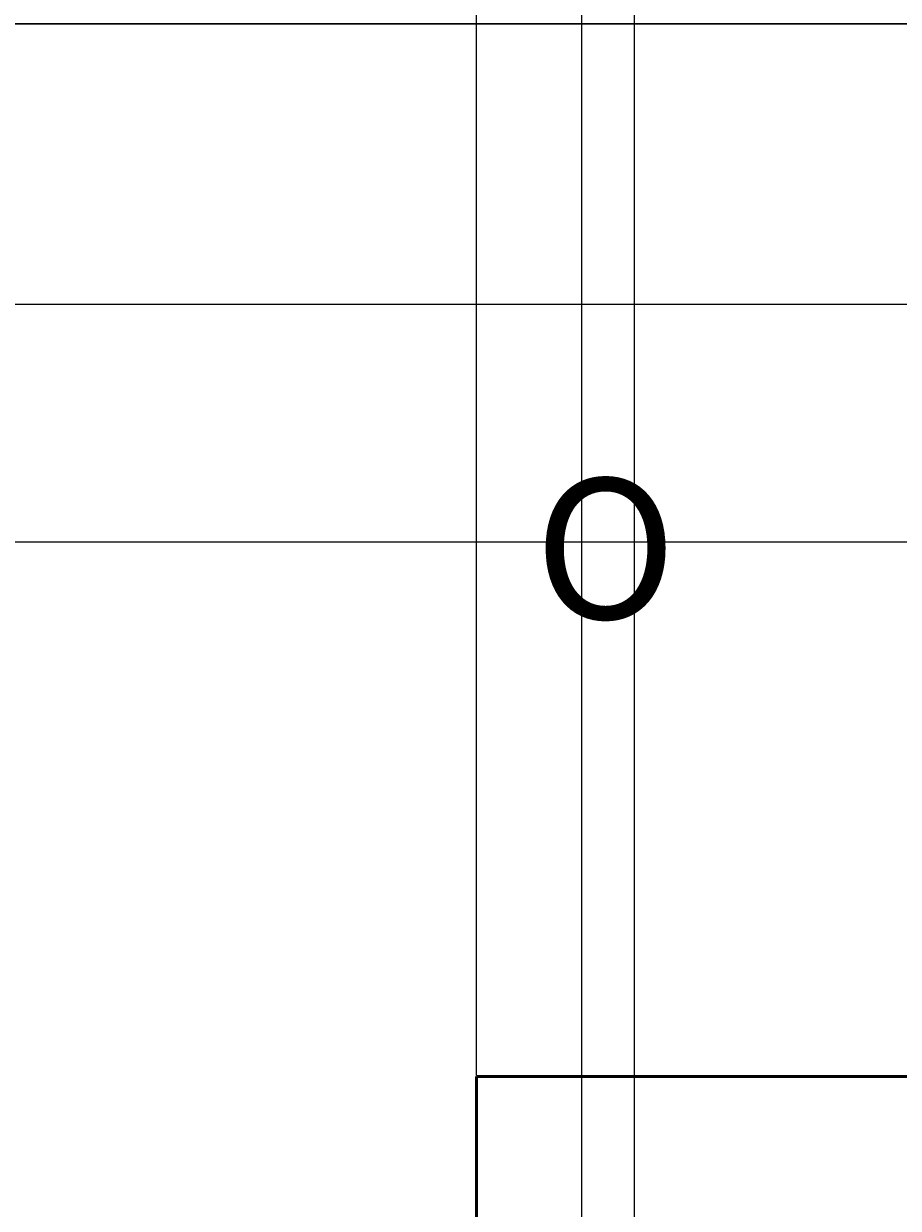
# Model space of a CAD drawing. Units: inches. Extents: x 37 to 824, y -700 to 234.
# Tile 63 of 77: x 264 to 314, y 8 to 75. Entities that reach past the tile are written whole.
import ezdxf

# ---------------------------------------------------------------- set-up
doc = ezdxf.new("R2010")
doc.units = ezdxf.units.IN
doc.header["$MEASUREMENT"] = 0
for name, color, linetype, lineweight in [('A-ANNO-DIMS', 2, 'Continuous', 18), ('A-ANNO-TEXT', 7, 'Continuous', 18), ('A-WALL', 2, 'Continuous', 50)]:
    doc.layers.add(name, color=color, linetype=linetype, lineweight=lineweight)
doc.styles.get("Standard").update_dxf_attribs({"font": 'arial.ttf'})
doc.dimstyles.get("Standard").update_dxf_attribs({"dimtxt": 0.18, "dimasz": 0.18, "dimexe": 0.18, "dimexo": 0.0625, "dimgap": 0.09, "dimtad": 0, "dimtih": 1, "dimtoh": 1, "dimdec": 1, "dimzin": 0, "dimdsep": 46, "dimlunit": 4, "dimtxsty": 'Standard', "dimcen": 0.09, "dimadec": 0, "dimazin": 0, "dimtfac": 1, "dimtdec": 1, "dimtofl": 0, "dimtmove": 0, "dimatfit": 3, "dimfxl": 1, "dimtolj": 1, "dimtzin": 0, "dimarcsym": 0})

# ---------------------------------------------------------------- blocks, each defined once
blk = doc.blocks.new('*D61')
at = {"layer": 'A-ANNO-DIMS', "color": 0, "lineweight": -2, "ltscale": 0.5, "transparency": 16777216}
for p, q in [((419.015, 75.09), (78.159, 75.09)), ((78.339, 74.91), (78.339, 67.271)), ((78.339, 59.27), (78.339, 66.91)), ((419.015, 59.09), (78.159, 59.09))]:
    blk.add_line(p, q, dxfattribs=at)
at = {"layer": 'A-ANNO-DIMS', "color": 0, "ltscale": 0.5, "transparency": 16777216}
for points in [[(78.309, 74.91), (78.369, 74.91), (78.339, 75.09)], [(78.309, 59.27), (78.369, 59.27), (78.339, 59.09)]]:
    blk.add_solid(points, dxfattribs=at)
at = {"layer": 'Defpoints', "color": 0, "ltscale": 0.5, "transparency": 16777216}
for p in [(419.077, 75.09), (78.339, 59.09), (419.077, 59.09)]:
    blk.add_point(p, dxfattribs=at)
at = {"layer": 'A-ANNO-DIMS', "color": 0, "ltscale": 0.5, "transparency": 16777216, "insert": (78.339, 67.09), "char_height": 0.18, "attachment_point": 5}
blk.add_mtext('\\A1;1\'-4"', dxfattribs=at)
blk = doc.blocks.new('*D76')
at = {"layer": 'A-ANNO-DIMS', "color": 0, "lineweight": -2, "ltscale": 0.5, "transparency": 16777216}
for p, q in [((227.14, 75.09), (513.773, 75.09)), ((513.593, 74.91), (513.593, 60.51)), ((513.593, 45.743), (513.593, 60.144)), ((227.14, 45.563), (513.773, 45.563))]:
    blk.add_line(p, q, dxfattribs=at)
at = {"layer": 'A-ANNO-DIMS', "color": 0, "ltscale": 0.5, "transparency": 16777216}
for points in [[(513.563, 74.91), (513.623, 74.91), (513.593, 75.09)], [(513.563, 45.743), (513.623, 45.743), (513.593, 45.563)]]:
    blk.add_solid(points, dxfattribs=at)
at = {"layer": 'Defpoints', "color": 0, "ltscale": 0.5, "transparency": 16777216}
for p in [(227.077, 75.09), (227.077, 45.563), (513.593, 45.563)]:
    blk.add_point(p, dxfattribs=at)
at = {"layer": 'A-ANNO-DIMS', "color": 0, "ltscale": 0.5, "transparency": 16777216, "insert": (513.593, 60.327), "char_height": 0.18, "attachment_point": 5}
blk.add_mtext('\\A1;2\'-5 1/2"', dxfattribs=at)
blk = doc.blocks.new('*D77')
at = {"layer": 'A-ANNO-DIMS', "color": 0, "lineweight": -2, "ltscale": 0.5, "transparency": 16777216}
for p, q in [((227.077, 45.5), (227.077, -400.406)), ((290.077, 15.028), (290.077, -400.406)), ((227.257, -400.226), (258.248, -400.226)), ((289.897, -400.226), (258.906, -400.226))]:
    blk.add_line(p, q, dxfattribs=at)
at = {"layer": 'A-ANNO-DIMS', "color": 0, "ltscale": 0.5, "transparency": 16777216}
for points in [[(227.257, -400.196), (227.257, -400.256), (227.077, -400.226)], [(289.897, -400.196), (289.897, -400.256), (290.077, -400.226)]]:
    blk.add_solid(points, dxfattribs=at)
at = {"layer": 'Defpoints', "color": 0, "ltscale": 0.5, "transparency": 16777216}
for p in [(227.077, 45.563), (290.077, 15.09), (290.077, -400.226)]:
    blk.add_point(p, dxfattribs=at)
at = {"layer": 'A-ANNO-DIMS', "color": 0, "ltscale": 0.5, "transparency": 16777216, "insert": (258.577, -400.226), "char_height": 0.18, "attachment_point": 5}
blk.add_mtext('\\A1;5\'-3"', dxfattribs=at)
blk = doc.blocks.new('*D78')
at = {"layer": 'A-ANNO-DIMS', "color": 0, "lineweight": -2, "ltscale": 0.5, "transparency": 16777216}
for p, q in [((290.077, 15.153), (290.077, 234.17)), ((290.257, 233.99), (325.747, 233.99)), ((361.897, 233.99), (326.407, 233.99)), ((362.077, 15.153), (362.077, 234.17))]:
    blk.add_line(p, q, dxfattribs=at)
at = {"layer": 'A-ANNO-DIMS', "color": 0, "ltscale": 0.5, "transparency": 16777216}
for points in [[(290.257, 234.02), (290.257, 233.96), (290.077, 233.99)], [(361.897, 234.02), (361.897, 233.96), (362.077, 233.99)]]:
    blk.add_solid(points, dxfattribs=at)
at = {"layer": 'Defpoints', "color": 0, "ltscale": 0.5, "transparency": 16777216}
for p in [(362.077, 233.99), (290.077, 15.09), (362.077, 15.09)]:
    blk.add_point(p, dxfattribs=at)
at = {"layer": 'A-ANNO-DIMS', "color": 0, "ltscale": 0.5, "transparency": 16777216, "insert": (326.077, 233.99), "char_height": 0.18, "attachment_point": 5}
blk.add_mtext('\\A1;6\'-0"', dxfattribs=at)
blk = doc.blocks.new('*D82')
at = {"layer": 'A-ANNO-DIMS', "color": 0, "lineweight": -2, "ltscale": 0.5, "transparency": 16777216}
for p, q in [((299.077, -206.847), (299.077, 234.17)), ((299.257, 233.99), (328.202, 233.99)), ((357.952, 233.99), (329.008, 233.99)), ((358.132, -206.847), (358.132, 234.17))]:
    blk.add_line(p, q, dxfattribs=at)
at = {"layer": 'A-ANNO-DIMS', "color": 0, "ltscale": 0.5, "transparency": 16777216}
for points in [[(299.257, 234.02), (299.257, 233.96), (299.077, 233.99)], [(357.952, 234.02), (357.952, 233.96), (358.132, 233.99)]]:
    blk.add_solid(points, dxfattribs=at)
at = {"layer": 'Defpoints', "color": 0, "ltscale": 0.5, "transparency": 16777216}
for p in [(358.132, 233.99), (299.077, -206.91), (358.132, -206.91)]:
    blk.add_point(p, dxfattribs=at)
at = {"layer": 'A-ANNO-DIMS', "color": 0, "ltscale": 0.5, "transparency": 16777216, "insert": (328.605, 233.99), "char_height": 0.18, "attachment_point": 5}
blk.add_mtext('\\A1;4\'-11"', dxfattribs=at)
blk = doc.blocks.new('*D87')
at = {"layer": 'A-ANNO-DIMS', "color": 0, "lineweight": -2, "ltscale": 0.5, "transparency": 16777216}
for p, q in [((216.077, -356.847), (216.077, 234.17)), ((216.257, 233.99), (255.747, 233.99)), ((295.897, 233.99), (256.407, 233.99)), ((296.077, -356.847), (296.077, 234.17))]:
    blk.add_line(p, q, dxfattribs=at)
at = {"layer": 'A-ANNO-DIMS', "color": 0, "ltscale": 0.5, "transparency": 16777216}
for points in [[(216.257, 234.02), (216.257, 233.96), (216.077, 233.99)], [(295.897, 234.02), (295.897, 233.96), (296.077, 233.99)]]:
    blk.add_solid(points, dxfattribs=at)
at = {"layer": 'Defpoints', "color": 0, "ltscale": 0.5, "transparency": 16777216}
for p in [(296.077, 233.99), (216.077, -356.91), (296.077, -356.91)]:
    blk.add_point(p, dxfattribs=at)
at = {"layer": 'A-ANNO-DIMS', "color": 0, "ltscale": 0.5, "transparency": 16777216, "insert": (256.077, 233.99), "char_height": 0.18, "attachment_point": 5}
blk.add_mtext('\\A1;6\'-8"', dxfattribs=at)

msp = doc.modelspace()

# ---------------------------------------------------------------- linework, layer by layer
at = {"layer": 'A-WALL'}
for p in [(362.077, 15.09), (290.077, -61.91)]:
    msp.add_line(p, (290.077, 15.09), dxfattribs=at)

# ---------------------------------------------------------------- texts
at = {"layer": 'A-ANNO-TEXT'}
msp.add_text('O', height=8, dxfattribs=at).set_placement((293.379, 41.174))

# ---------------------------------------------------------------- dimensions: what is measured, and where the dimension line sits
at = {"layer": 'A-ANNO-DIMS', "ltscale": 0.5}
for base, p1, p2, picture, middle in [((296.077, 233.99), (216.077, -356.91), (296.077, -356.91), '*D87', (256.077, 233.99)), ((362.077, 233.99), (290.077, 15.09), (362.077, 15.09), '*D78', (326.077, 233.99)), ((358.132, 233.99), (299.077, -206.91), (358.132, -206.91), '*D82', (328.605, 233.99)), ((290.077, -400.226), (227.077, 45.563), (290.077, 15.09), '*D77', (258.577, -400.226))]:
    dim = msp.add_linear_dim(base=base, p1=p1, p2=p2, dimstyle='Standard', override={"dimdec": 1, "dimlfac": 1, "dimrnd": 0, "dimzin": 1, "dimdsep": 46, "dimlunit": 4, "dimfrac": 2}, dxfattribs=at)
    dim.commit()
    dim.dimension.update_dxf_attribs({"geometry": picture, "text_midpoint": middle})
for base, p1, p2, picture, middle in [((78.339, 59.09), (419.077, 75.09), (419.077, 59.09), '*D61', (78.339, 67.09)), ((513.593, 45.563), (227.077, 75.09), (227.077, 45.563), '*D76', (513.593, 60.327))]:
    dim = msp.add_linear_dim(base=base, p1=p1, p2=p2, angle=90, dimstyle='Standard', override={"dimdec": 1, "dimlfac": 1, "dimrnd": 0, "dimzin": 1, "dimdsep": 46, "dimlunit": 4, "dimfrac": 2}, dxfattribs=at)
    dim.commit()
    dim.dimension.update_dxf_attribs({"geometry": picture, "text_midpoint": middle})

doc.saveas('drawing.dxf')
